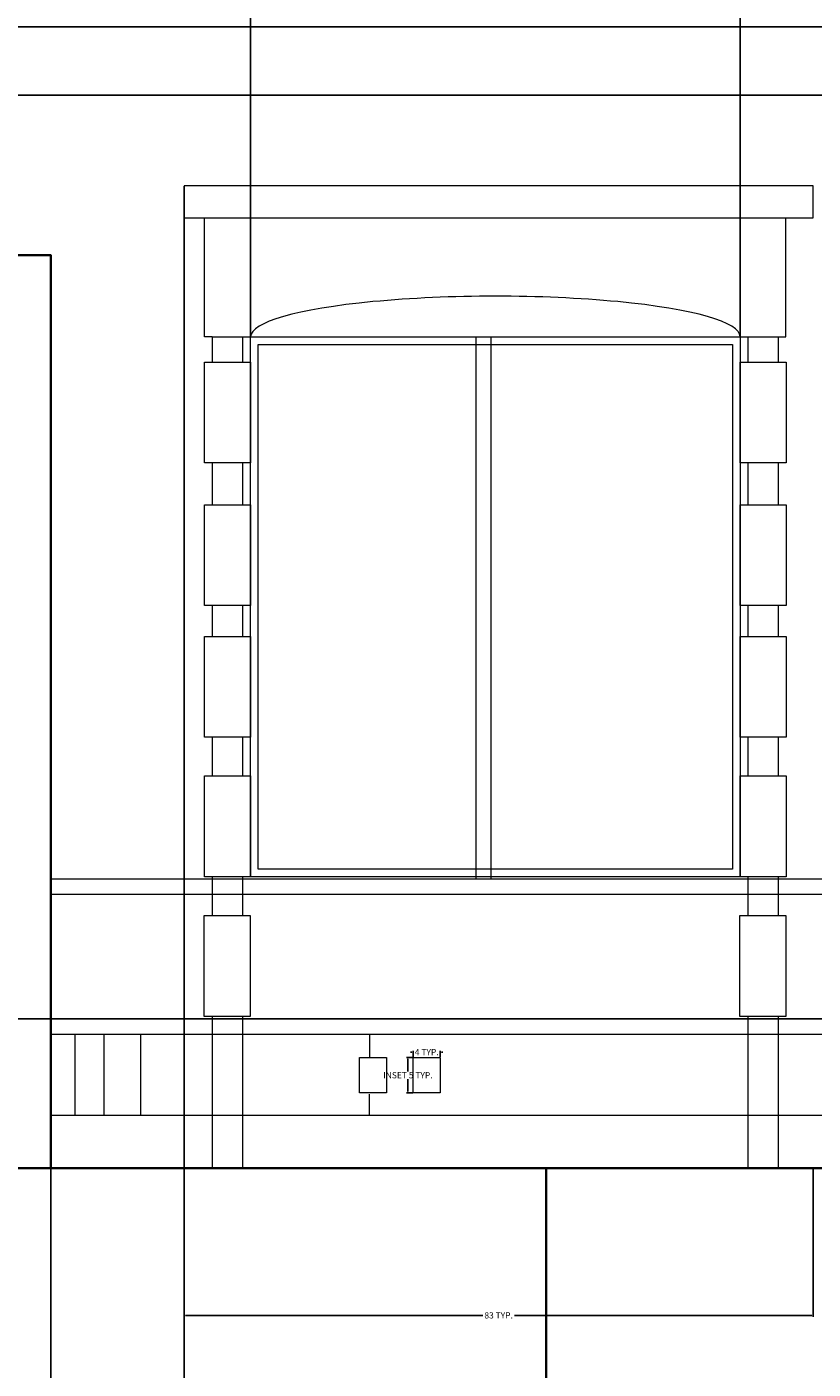
# Model space of a CAD drawing. Units: inches. Extents: x 69 to 650, y -16 to 573.
# Tile 13 of 26: x 187 to 290, y 218 to 394. Entities that reach past the tile are written whole.
import ezdxf

# ---------------------------------------------------------------- set-up
doc = ezdxf.new("R2010")
doc.units = ezdxf.units.IN
doc.header["$MEASUREMENT"] = 0
for name, color, linetype, lineweight in [('A-ANNO-DIMS', 2, 'Continuous', 18), ('A-ELEV', 8, 'Continuous', 18), ('A-GLAZ', 4, 'Continuous', 18), ('A-WALL', 7, 'Continuous', 35)]:
    doc.layers.add(name, color=color, linetype=linetype, lineweight=lineweight)
doc.styles.get("Standard").update_dxf_attribs({"font": 'arial.ttf'})
doc.dimstyles.get("Standard").update_dxf_attribs({"dimtxt": 0.8125, "dimasz": 0.18, "dimexe": 0.18, "dimexo": 0.0625, "dimgap": 0.09, "dimtad": 0, "dimtih": 1, "dimtoh": 1, "dimdec": 4, "dimzin": 0, "dimdsep": 46, "dimlunit": 4, "dimtxsty": 'Standard', "dimcen": 0.09, "dimadec": 0, "dimazin": 0, "dimtfac": 1, "dimtdec": 4, "dimtofl": 0, "dimtmove": 0, "dimatfit": 3, "dimfxl": 1, "dimtolj": 1, "dimtzin": 0, "dimarcsym": 0})

# ---------------------------------------------------------------- blocks, each defined once
blk = doc.blocks.new('WIN-ARCH-SURROUND')
for p, q in [((0, 129.06), (0, 124.83)), ((82.63, 129.06), (0, 129.06)), ((82.63, 124.83), (82.63, 129.06)), ((0, 124.83), (82.63, 124.83)), ((2.69, 109.21), (2.69, 124.83)), ((79.05, 109.21), (79.05, 124.83)), ((3.69, 109.21), (2.69, 109.21)), ((3.69, 109.21), (3.69, 105.89)), ((3.69, 109.21), (78.05, 109.21)), ((7.69, 109.21), (7.69, 105.89)), ((8.73, 105.89), (8.73, 109.21)), ((38.31, 109.21), (38.31, 38)), ((40.31, 109.21), (40.31, 38)), ((74.05, 109.21), (74.05, 105.89)), ((78.05, 109.21), (79.05, 109.21)), ((78.05, 109.21), (78.05, 105.89)), ((3.69, 92.64), (3.69, 87.15)), ((7.69, 92.64), (7.69, 87.15)), ((74.05, 92.64), (74.05, 87.15)), ((78.05, 92.64), (78.05, 87.15)), ((3.69, 73.9), (3.69, 69.84)), ((7.69, 73.9), (7.69, 69.84)), ((74.05, 73.9), (74.05, 69.84)), ((78.05, 73.9), (78.05, 69.84)), ((3.69, 56.59), (3.69, 51.51)), ((7.69, 56.59), (7.69, 51.51)), ((74.05, 56.59), (74.05, 51.51)), ((78.05, 56.59), (78.05, 51.51)), ((3.69, 38.26), (3.69, 33.16)), ((7.69, 38.26), (7.69, 33.16)), ((74.05, 38.26), (74.05, 33.16)), ((78.05, 38.26), (78.05, 33.16)), ((3.69, 19.91), (3.69, 0)), ((7.69, 19.91), (7.69, 0)), ((74.05, 19.91), (74.05, 0)), ((78.05, 19.91), (78.05, 0))]:
    blk.add_line(p, q)
for points in [[(8.73, 109.21), (73.05, 109.21), (73.05, 38.26), (8.73, 38.26)], [(9.73, 108.21), (72.05, 108.21), (72.05, 39.26), (9.73, 39.26)], [(2.69, 105.89), (8.73, 105.89), (8.73, 92.64), (2.69, 92.64)], [(73.05, 105.89), (79.1, 105.89), (79.1, 92.64), (73.05, 92.64)], [(2.69, 87.15), (8.73, 87.15), (8.73, 73.9), (2.69, 73.9)], [(73.05, 87.15), (79.1, 87.15), (79.1, 73.9), (73.05, 73.9)], [(2.69, 69.84), (8.73, 69.84), (8.73, 56.59), (2.69, 56.59)], [(73.05, 69.84), (79.1, 69.84), (79.1, 56.59), (73.05, 56.59)], [(2.69, 51.51), (8.73, 51.51), (8.73, 38.26), (2.69, 38.26)], [(73.05, 51.51), (79.1, 51.51), (79.1, 38.26), (73.05, 38.26)], [(2.65, 33.16), (8.69, 33.16), (8.69, 19.91), (2.65, 19.91)], [(73.01, 33.16), (79.06, 33.16), (79.06, 19.91), (73.01, 19.91)]]:
    blk.add_lwpolyline(points, close=True)
blk.add_ellipse((40.89, 109.21), major_axis=(32.16, 0), ratio=0.165597, start_param=6.283185, end_param=9.424778)
blk = doc.blocks.new('TRIM-FRIEZE-INSET')
blk.add_lwpolyline([(0, 4.66), (3.54, 4.66), (3.54, 0), (0, 0)], close=True)
blk = doc.blocks.new('*D9')
at = {"layer": 'A-ANNO-DIMS', "color": 0, "lineweight": -2, "transparency": 16777216}
for p, q in [((237.85, 258.46), (237.04, 258.46)), ((237.22, 258.28), (237.22, 256.63)), ((237.22, 253.97), (237.22, 255.61)), ((237.85, 253.79), (237.04, 253.79))]:
    blk.add_line(p, q, dxfattribs=at)
at = {"layer": 'A-ANNO-DIMS', "color": 0, "transparency": 16777216}
for points in [[(237.19, 258.28), (237.25, 258.28), (237.22, 258.46)], [(237.19, 253.97), (237.25, 253.97), (237.22, 253.79)]]:
    blk.add_solid(points, dxfattribs=at)
at = {"layer": 'Defpoints', "color": 0, "transparency": 16777216}
for p in [(237.22, 258.46), (237.92, 258.46), (237.92, 253.79)]:
    blk.add_point(p, dxfattribs=at)
at = {"layer": 'A-ANNO-DIMS', "color": 0, "transparency": 16777216, "insert": (237.22, 256.12), "char_height": 0.8125, "attachment_point": 5}
blk.add_mtext('\\A1;INSET 5 TYP.', dxfattribs=at)
blk = doc.blocks.new('*D10')
at = {"layer": 'A-ANNO-DIMS', "color": 0, "lineweight": -2, "transparency": 16777216}
for p, q in [((237.92, 258.52), (237.92, 259.34)), ((241.45, 258.52), (241.45, 259.34)), ((237.74, 259.16), (237.56, 259.16)), ((241.63, 259.16), (241.81, 259.16))]:
    blk.add_line(p, q, dxfattribs=at)
at = {"layer": 'A-ANNO-DIMS', "color": 0, "transparency": 16777216}
for points in [[(237.74, 259.19), (237.74, 259.13), (237.92, 259.16)], [(241.63, 259.19), (241.63, 259.13), (241.45, 259.16)]]:
    blk.add_solid(points, dxfattribs=at)
at = {"layer": 'Defpoints', "color": 0, "transparency": 16777216}
for p in [(237.92, 258.46), (241.45, 259.16), (241.45, 258.46)]:
    blk.add_point(p, dxfattribs=at)
at = {"layer": 'A-ANNO-DIMS', "color": 0, "transparency": 16777216, "insert": (239.69, 259.16), "char_height": 0.812, "attachment_point": 5}
blk.add_mtext('\\A1;4 TYP.', dxfattribs=at)
blk = doc.blocks.new('*D14')
at = {"layer": 'A-ANNO-DIMS', "color": 0, "lineweight": -2, "transparency": 16777216}
for p, q in [((207.81, 243.87), (207.81, 224.39)), ((290.45, 243.87), (290.45, 224.39)), ((207.99, 224.57), (247.06, 224.57)), ((290.27, 224.57), (251.2, 224.57))]:
    blk.add_line(p, q, dxfattribs=at)
at = {"layer": 'A-ANNO-DIMS', "color": 0, "transparency": 16777216}
for points in [[(207.99, 224.6), (207.99, 224.54), (207.81, 224.57)], [(290.27, 224.6), (290.27, 224.54), (290.45, 224.57)]]:
    blk.add_solid(points, dxfattribs=at)
at = {"layer": 'Defpoints', "color": 0, "transparency": 16777216}
for p in [(207.81, 243.93), (290.45, 243.93), (290.45, 224.57)]:
    blk.add_point(p, dxfattribs=at)
at = {"layer": 'A-ANNO-DIMS', "color": 0, "transparency": 16777216, "insert": (249.13, 224.57), "char_height": 0.8125, "attachment_point": 5}
blk.add_mtext('\\A1;83 TYP.', dxfattribs=at)
blk = doc.blocks.new('*D19')
at = {"layer": 'A-ANNO-DIMS', "color": 0, "lineweight": -2, "transparency": 16777216}
for p, q in [((99.56, 471.72), (99.56, 572.74)), ((99.74, 572.56), (358.57, 572.56)), ((619.38, 572.56), (360.54, 572.56)), ((619.56, 87.99), (619.56, 572.74))]:
    blk.add_line(p, q, dxfattribs=at)
at = {"layer": 'A-ANNO-DIMS', "color": 0, "transparency": 16777216}
for points in [[(99.74, 572.59), (99.74, 572.53), (99.56, 572.56)], [(619.38, 572.59), (619.38, 572.53), (619.56, 572.56)]]:
    blk.add_solid(points, dxfattribs=at)
at = {"layer": 'Defpoints', "color": 0, "transparency": 16777216}
for p in [(619.56, 572.56), (99.56, 471.66), (619.56, 87.93)]:
    blk.add_point(p, dxfattribs=at)
at = {"layer": 'A-ANNO-DIMS', "color": 0, "transparency": 16777216, "insert": (359.56, 572.56), "char_height": 0.812, "attachment_point": 5}
blk.add_mtext('\\A1;520', dxfattribs=at)
blk = doc.blocks.new('*D25')
at = {"layer": 'A-ANNO-DIMS', "color": 0, "lineweight": -2, "transparency": 16777216}
for p, q in [((99.49, 243.93), (70.98, 243.93)), ((71.16, 243.75), (71.16, 228.3)), ((71.16, 211.83), (71.16, 227.29)), ((441.88, 211.65), (70.98, 211.65))]:
    blk.add_line(p, q, dxfattribs=at)
at = {"layer": 'A-ANNO-DIMS', "color": 0, "transparency": 16777216}
for points in [[(71.13, 243.75), (71.19, 243.75), (71.16, 243.93)], [(71.13, 211.83), (71.19, 211.83), (71.16, 211.65)]]:
    blk.add_solid(points, dxfattribs=at)
at = {"layer": 'Defpoints', "color": 0, "transparency": 16777216}
for p in [(71.16, 243.93), (99.56, 243.93), (441.94, 211.65)]:
    blk.add_point(p, dxfattribs=at)
at = {"layer": 'A-ANNO-DIMS', "color": 0, "transparency": 16777216, "insert": (71.16, 227.79), "char_height": 0.812, "attachment_point": 5}
blk.add_mtext('\\A1;32.28', dxfattribs=at)
blk = doc.blocks.new('*D35')
at = {"layer": 'A-ANNO-DIMS', "color": 0, "lineweight": -2, "transparency": 16777216}
for p, q in [((99.56, 243.87), (99.56, 35.35)), ((190.3, 243.87), (190.3, 35.35)), ((99.74, 35.53), (143.47, 35.53)), ((190.12, 35.53), (146.39, 35.53))]:
    blk.add_line(p, q, dxfattribs=at)
at = {"layer": 'A-ANNO-DIMS', "color": 0, "transparency": 16777216}
for points in [[(99.74, 35.56), (99.74, 35.5), (99.56, 35.53)], [(190.12, 35.56), (190.12, 35.5), (190.3, 35.53)]]:
    blk.add_solid(points, dxfattribs=at)
at = {"layer": 'Defpoints', "color": 0, "transparency": 16777216}
for p in [(99.56, 243.93), (190.3, 243.93), (190.3, 35.53)]:
    blk.add_point(p, dxfattribs=at)
at = {"layer": 'A-ANNO-DIMS', "color": 0, "transparency": 16777216, "insert": (144.93, 35.53), "char_height": 0.812, "attachment_point": 5}
blk.add_mtext('\\A1;90.74', dxfattribs=at)
blk = doc.blocks.new('*D36')
at = {"layer": 'A-ANNO-DIMS', "color": 0, "lineweight": -2, "transparency": 16777216}
for p, q in [((207.81, 372.93), (207.81, 35.35)), ((190.3, 243.87), (190.3, 35.35)), ((190.48, 35.53), (197.32, 35.53)), ((207.63, 35.53), (200.79, 35.53))]:
    blk.add_line(p, q, dxfattribs=at)
at = {"layer": 'A-ANNO-DIMS', "color": 0, "transparency": 16777216}
for points in [[(190.48, 35.56), (190.48, 35.5), (190.3, 35.53)], [(207.63, 35.56), (207.63, 35.5), (207.81, 35.53)]]:
    blk.add_solid(points, dxfattribs=at)
at = {"layer": 'Defpoints', "color": 0, "transparency": 16777216}
for p in [(207.81, 372.99), (190.3, 243.93), (207.81, 35.53)]:
    blk.add_point(p, dxfattribs=at)
at = {"layer": 'A-ANNO-DIMS', "color": 0, "transparency": 16777216, "insert": (199.06, 35.53), "char_height": 0.812, "attachment_point": 5}
blk.add_mtext('\\A1;17.514', dxfattribs=at)
blk = doc.blocks.new('*D45')
at = {"layer": 'A-ANNO-DIMS', "color": 0, "lineweight": -2, "transparency": 16777216}
for p, q in [((216.55, 353.2), (216.55, 572.74)), ((216.73, 572.56), (247.25, 572.56)), ((280.68, 572.56), (250.16, 572.56)), ((280.86, 353.2), (280.86, 572.74))]:
    blk.add_line(p, q, dxfattribs=at)
at = {"layer": 'A-ANNO-DIMS', "color": 0, "transparency": 16777216}
for points in [[(216.73, 572.59), (216.73, 572.53), (216.55, 572.56)], [(280.68, 572.59), (280.68, 572.53), (280.86, 572.56)]]:
    blk.add_solid(points, dxfattribs=at)
at = {"layer": 'Defpoints', "color": 0, "transparency": 16777216}
for p in [(280.86, 572.56), (216.55, 353.14), (280.86, 353.14)]:
    blk.add_point(p, dxfattribs=at)
at = {"layer": 'A-ANNO-DIMS', "color": 0, "transparency": 16777216, "insert": (248.71, 572.56), "char_height": 0.812, "attachment_point": 5}
blk.add_mtext('\\A1;64.32', dxfattribs=at)
blk = doc.blocks.new('*D58')
at = {"layer": 'A-ANNO-DIMS', "color": 0, "lineweight": -2, "transparency": 16777216}
for p, q in [((313.74, 263.53), (70.98, 263.53)), ((71.16, 263.35), (71.16, 254.23)), ((71.16, 244.11), (71.16, 253.22)), ((190.24, 243.93), (70.98, 243.93))]:
    blk.add_line(p, q, dxfattribs=at)
at = {"layer": 'A-ANNO-DIMS', "color": 0, "transparency": 16777216}
for points in [[(71.13, 263.35), (71.19, 263.35), (71.16, 263.53)], [(71.13, 244.11), (71.19, 244.11), (71.16, 243.93)]]:
    blk.add_solid(points, dxfattribs=at)
at = {"layer": 'Defpoints', "color": 0, "transparency": 16777216}
for p in [(71.16, 263.53), (313.81, 263.53), (190.3, 243.93)]:
    blk.add_point(p, dxfattribs=at)
at = {"layer": 'A-ANNO-DIMS', "color": 0, "transparency": 16777216, "insert": (71.16, 253.73), "char_height": 0.812, "attachment_point": 5}
blk.add_mtext('\\A1;19.595', dxfattribs=at)
blk = doc.blocks.new('*D59')
at = {"layer": 'A-ANNO-DIMS', "color": 0, "lineweight": -2, "transparency": 16777216}
for p, q in [((214.82, 402.3), (70.98, 402.3)), ((71.16, 402.12), (71.16, 394.11)), ((71.16, 385.08), (71.16, 393.1)), ((307.73, 384.9), (70.98, 384.9))]:
    blk.add_line(p, q, dxfattribs=at)
at = {"layer": 'A-ANNO-DIMS', "color": 0, "transparency": 16777216}
for points in [[(71.13, 402.12), (71.19, 402.12), (71.16, 402.3)], [(71.13, 385.08), (71.19, 385.08), (71.16, 384.9)]]:
    blk.add_solid(points, dxfattribs=at)
at = {"layer": 'Defpoints', "color": 0, "transparency": 16777216}
for p in [(71.16, 402.3), (214.89, 402.3), (307.8, 384.9)]:
    blk.add_point(p, dxfattribs=at)
at = {"layer": 'A-ANNO-DIMS', "color": 0, "transparency": 16777216, "insert": (71.16, 393.6), "char_height": 0.812, "attachment_point": 5}
blk.add_mtext('\\A1;17.406', dxfattribs=at)
blk = doc.blocks.new('*D63')
at = {"layer": 'A-ANNO-DIMS', "color": 0, "lineweight": -2, "transparency": 16777216}
for p, q in [((319.49, 393.86), (70.98, 393.86)), ((71.16, 393.68), (71.16, 389.88)), ((71.16, 385.08), (71.16, 388.87)), ((307.73, 384.9), (70.98, 384.9))]:
    blk.add_line(p, q, dxfattribs=at)
at = {"layer": 'A-ANNO-DIMS', "color": 0, "transparency": 16777216}
for points in [[(71.13, 393.68), (71.19, 393.68), (71.16, 393.86)], [(71.13, 385.08), (71.19, 385.08), (71.16, 384.9)]]:
    blk.add_solid(points, dxfattribs=at)
at = {"layer": 'Defpoints', "color": 0, "transparency": 16777216}
for p in [(71.16, 393.86), (319.55, 393.86), (307.8, 384.9)]:
    blk.add_point(p, dxfattribs=at)
at = {"layer": 'A-ANNO-DIMS', "color": 0, "transparency": 16777216, "insert": (71.16, 389.38), "char_height": 0.812, "attachment_point": 5}
blk.add_mtext('\\A1;8.959', dxfattribs=at)

msp = doc.modelspace()

# ---------------------------------------------------------------- linework, layer by layer
at = {"layer": 'A-ELEV'}
for p, q in [((190.299, 281.93), (528.812, 281.93)), ((190.299, 279.93), (528.812, 279.93)), ((190.299, 263.5253), (528.812, 263.5253)), ((190.299, 261.5253), (528.812, 261.5253)), ((193.4702, 261.5253), (193.4702, 250.8759)), ((197.2942, 261.5253), (197.2942, 250.8759)), ((202.0851, 261.5253), (202.0851, 250.8759)), ((232.188, 261.5253), (232.188, 258.386)), ((232.188, 250.8759), (232.188, 253.6508)), ((190.299, 250.8759), (484.5159, 250.8759))]:
    msp.add_line(p, q, dxfattribs=at)
at = {"layer": 'A-WALL'}
for p, q in [((99.556, 243.93), (619.555, 243.93)), ((255.3778, 243.93), (255.3778, 87.93))]:
    msp.add_line(p, q, dxfattribs=at)
msp.add_lwpolyline([(99.556, 363.8739), (190.299, 363.8739), (190.299, 243.93), (99.556, 243.93)], close=True, dxfattribs=at)

# ---------------------------------------------------------------- block references
at = {"layer": 'A-ELEV'}
for p in [(230.844, 253.792), (237.9171, 253.792)]:
    msp.add_blockref('TRIM-FRIEZE-INSET', p, dxfattribs=at)
at = {"layer": 'A-GLAZ'}
msp.add_blockref('WIN-ARCH-SURROUND', (207.813, 243.93), dxfattribs=at)

# ---------------------------------------------------------------- dimensions: what is measured, and where the dimension line sits
at = {"layer": 'A-ANNO-DIMS'}
for base, p1, p2, override, picture, middle in [((619.555, 572.5573), (99.556, 471.6595), (619.555, 87.93), {"dimdec": 0, "dimlfac": 1, "dimrnd": 0, "dimzin": 0, "dimdsep": 46, "dimlunit": 2}, '*D19', (359.5555, 572.5573)), ((280.864, 572.5573), (216.5473, 353.1381), (280.864, 353.1381), {"dimdec": 2, "dimlfac": 1, "dimrnd": 0, "dimzin": 0, "dimdsep": 46, "dimlunit": 2}, '*D45', (248.7057, 572.5573)), ((207.8126, 35.53), (190.299, 243.93), (207.8126, 372.9907), {"dimdec": 3, "dimlfac": 1, "dimrnd": 0, "dimzin": 0, "dimdsep": 46, "dimlunit": 2}, '*D36', (199.0558, 35.53)), ((190.299, 35.53), (99.556, 243.93), (190.299, 243.93), {"dimdec": 2, "dimlfac": 1, "dimrnd": 0, "dimzin": 0, "dimdsep": 46, "dimlunit": 2}, '*D35', (144.9275, 35.53))]:
    dim = msp.add_linear_dim(base=base, p1=p1, p2=p2, dimstyle='Standard', override=override, dxfattribs=at)
    dim.commit()
    dim.dimension.update_dxf_attribs({"geometry": picture, "text_midpoint": middle})
for base, p1, p2, override, picture, middle in [((71.156, 402.3042), (307.7955, 384.8986), (214.8863, 402.3042), {"dimdec": 3, "dimlfac": 1, "dimrnd": 0, "dimzin": 0, "dimdsep": 46, "dimlunit": 2}, '*D59', (71.156, 393.6014)), ((71.156, 393.8576), (307.7955, 384.8986), (319.5513, 393.8576), {"dimdec": 3, "dimlfac": 1, "dimrnd": 0, "dimzin": 0, "dimdsep": 46, "dimlunit": 2}, '*D63', (71.156, 389.3781)), ((71.156, 263.5253), (190.299, 243.93), (313.8067, 263.5253), {"dimdec": 3, "dimlfac": 1, "dimrnd": 0, "dimzin": 0, "dimdsep": 46, "dimlunit": 2}, '*D58', (71.156, 253.7277)), ((71.156, 243.93), (441.9398, 211.6519), (99.556, 243.93), {"dimdec": 2, "dimlfac": 1, "dimrnd": 0, "dimzin": 0, "dimdsep": 46, "dimlunit": 2}, '*D25', (71.156, 227.7909))]:
    dim = msp.add_linear_dim(base=base, p1=p1, p2=p2, angle=90, dimstyle='Standard', override=override, dxfattribs=at)
    dim.commit()
    dim.dimension.update_dxf_attribs({"geometry": picture, "text_midpoint": middle})
for base, p1, p2, picture, middle in [((241.4539, 259.1564), (237.9173, 258.4567), (241.4539, 258.4567), '*D10', (239.6856, 259.1564)), ((290.4461, 224.5709), (207.8126, 243.93), (290.4461, 243.93), '*D14', (249.1293, 224.5709))]:
    dim = msp.add_linear_dim(base=base, p1=p1, p2=p2, text='<> TYP.', dimstyle='Standard', override={"dimdec": 0, "dimlfac": 1, "dimrnd": 0, "dimzin": 0, "dimdsep": 46, "dimlunit": 2}, dxfattribs=at)
    dim.commit()
    dim.dimension.update_dxf_attribs({"geometry": picture, "text_midpoint": middle})
dim = msp.add_linear_dim(base=(237.2176, 258.4567), p1=(237.9173, 253.7922), p2=(237.9173, 258.4567), angle=90, text='INSET <> TYP.', dimstyle='Standard', override={"dimdec": 0, "dimlfac": 1, "dimrnd": 0, "dimzin": 0, "dimdsep": 46, "dimlunit": 2}, dxfattribs=at)
dim.commit()
dim.dimension.update_dxf_attribs({"geometry": '*D9', "text_midpoint": (237.2176, 256.1245)})

doc.saveas('drawing.dxf')
